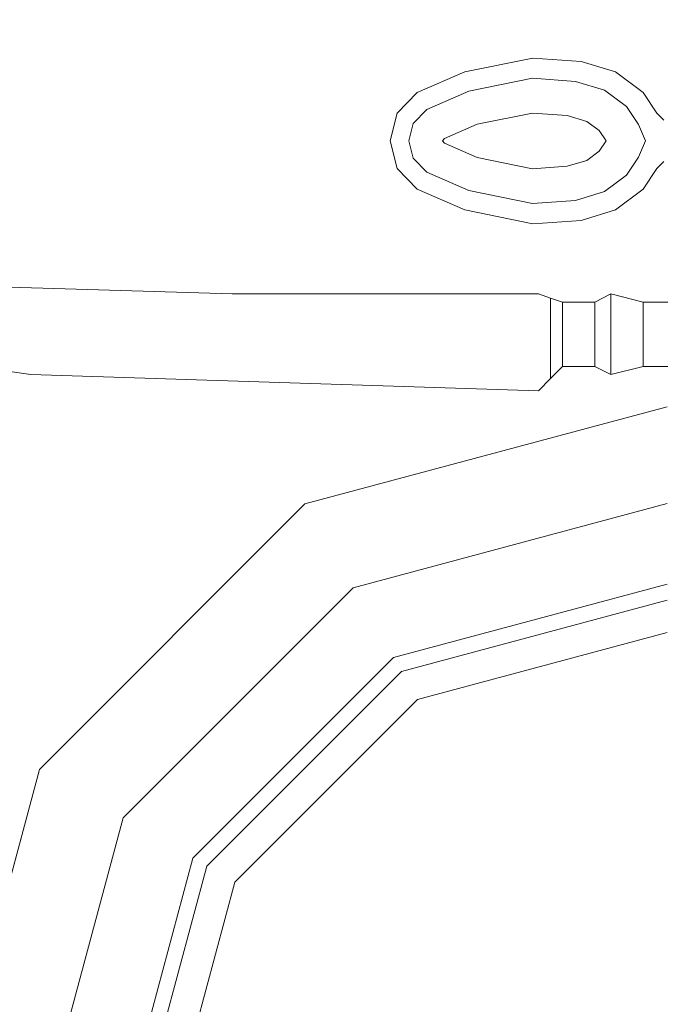
# Model space of a CAD drawing. Units: inches. Extents: x 375 to 1122, y 27 to 1069.
# Tile 62 of 155: x 734.823 to 739.718, y 304.063 to 311.585. Entities that reach past the tile are written whole.
import ezdxf

# ---------------------------------------------------------------- set-up
doc = ezdxf.new("R2010")
doc.units = ezdxf.units.IN
doc.layers.add('A-ANNO-DIMS', color=2, linetype='Continuous', lineweight=18)
doc.layers.add('Furniture', color=30, linetype='Continuous', lineweight=18)
doc.styles.get("Standard").update_dxf_attribs({"font": 'arial.ttf'})
doc.dimstyles.new('ISO-25', dxfattribs={"dimtxt": 12, "dimasz": 2.5, "dimexe": 1.5, "dimexo": 1.5, "dimtad": 1, "dimdec": 1, "dimlunit": 3, "dimtxsty": 'Standard', "dimblk": 'ARCHTICK', "dimcen": 2.5, "dimadec": 0, "dimazin": 0, "dimtfac": 1, "dimtdec": 1, "dimtmove": 0, "dimatfit": 3, "dimfxl": 1.5, "dimfxlon": 1, "dimarcsym": 0})

# ---------------------------------------------------------------- blocks, each defined once
blk = doc.blocks.new('A$C403C54AD')
for points, invisible_edges in [([(0.93398, 1.36607, -0.03581), (0.92167, 1.36607, -0.03581), (0.92167, 1.40455, -0.03427), (0.93398, 1.40455, -0.03427)], 4), ([(0.93398, 1.36607, -0.04504), (0.92167, 1.36607, -0.04504), (0.92167, 1.40455, -0.04658), (0.93398, 1.40455, -0.04658)], 4), ([(0.89484, 1.37003, -0.04027), (0.88693, 1.37003, -0.04027), (0.88561, 1.3687, -0.041), (0.89616, 1.3687, -0.041)], 5), ([(0.89484, 1.37003, -0.04236), (0.88693, 1.37003, -0.04236), (0.88561, 1.3687, -0.04315), (0.89616, 1.3687, -0.04315)], 5), ([(0.88693, 1.37003, -0.04236), (0.88693, 1.37003, -0.04027), (0.88561, 1.3687, -0.041), (0.88561, 1.3687, -0.04315)], 1), ([(0.89484, 1.37003, -0.04027), (0.89484, 1.37003, -0.04236), (0.89616, 1.3687, -0.04315), (0.89616, 1.3687, -0.041)], 1), ([(0.88774, 1.36518, -0.04424), (0.88561, 1.3687, -0.04315), (0.88165, 1.36608, -0.04195), (0.88434, 1.36289, -0.04423)], 5), ([(0.88774, 1.36518, -0.04292), (0.88561, 1.3687, -0.041), (0.88165, 1.36608, -0.04063), (0.88434, 1.36289, -0.04291)], 5), ([(0.88561, 1.3687, -0.04315), (0.89088, 1.3687, -0.04315), (0.89088, 1.36654, -0.04406), (0.88774, 1.36518, -0.04424)], 11), ([(0.88561, 1.3687, -0.041), (0.89088, 1.3687, -0.041), (0.89088, 1.36654, -0.04274), (0.88774, 1.36518, -0.04292)], 11), ([(0.89616, 1.3687, -0.04315), (0.89088, 1.3687, -0.04315), (0.89088, 1.36654, -0.04406), (0.89402, 1.36518, -0.04424)], 11), ([(0.89616, 1.3687, -0.041), (0.89088, 1.3687, -0.041), (0.89088, 1.36654, -0.04274), (0.89402, 1.36518, -0.04292)], 11), ([(0.89402, 1.36518, -0.04292), (0.89616, 1.3687, -0.041), (0.90012, 1.36608, -0.04063), (0.89743, 1.36289, -0.04291)], 5), ([(0.88165, 1.36608, -0.04195), (0.88434, 1.36289, -0.04423), (0.88119, 1.35867, -0.04406), (0.87769, 1.36082, -0.04147)], 5), ([(0.88165, 1.36608, -0.04063), (0.88434, 1.36289, -0.04291), (0.88119, 1.35867, -0.04274), (0.87769, 1.36082, -0.04015)], 5), ([(0.88774, 1.36518, -0.04424), (0.89088, 1.35902, -0.04627), (0.89088, 1.35902, -0.04627), (0.89088, 1.36654, -0.04406)], 5), ([(0.88774, 1.36518, -0.04292), (0.89088, 1.35902, -0.04495), (0.89088, 1.35902, -0.04495), (0.89088, 1.36654, -0.04274)], 5), ([(0.89402, 1.36518, -0.04424), (0.89088, 1.35902, -0.04627), (0.89088, 1.35902, -0.04627), (0.89088, 1.36654, -0.04406)], 5), ([(0.89402, 1.36518, -0.04292), (0.89088, 1.35902, -0.04495), (0.89088, 1.35902, -0.04495), (0.89088, 1.36654, -0.04274)], 5), ([(0.90012, 1.36608, -0.04195), (0.89743, 1.36289, -0.04423), (0.90058, 1.35867, -0.04406), (0.90408, 1.36082, -0.04147)], 5), ([(0.90012, 1.36608, -0.04063), (0.89743, 1.36289, -0.04291), (0.90058, 1.35867, -0.04274), (0.90408, 1.36082, -0.04015)], 5), ([(0.88892, 1.35767, -0.04647), (0.88434, 1.36289, -0.04423), (0.88774, 1.36518, -0.04424), (0.89088, 1.35902, -0.04627)], 5), ([(0.88892, 1.35767, -0.04515), (0.88434, 1.36289, -0.04291), (0.88774, 1.36518, -0.04292), (0.89088, 1.35902, -0.04495)], 5), ([(0.89284, 1.35767, -0.04647), (0.89743, 1.36289, -0.04423), (0.89402, 1.36518, -0.04424), (0.89088, 1.35902, -0.04627)], 5), ([(0.89284, 1.35767, -0.04515), (0.89743, 1.36289, -0.04291), (0.89402, 1.36518, -0.04292), (0.89088, 1.35902, -0.04495)], 5), ([(0.88119, 1.35867, -0.04406), (0.88715, 1.3553, -0.04638), (0.88892, 1.35767, -0.04647), (0.88434, 1.36289, -0.04423)], 5), ([(0.88119, 1.35867, -0.04274), (0.88715, 1.3553, -0.04506), (0.88892, 1.35767, -0.04515), (0.88434, 1.36289, -0.04291)], 5), ([(0.90058, 1.35867, -0.04406), (0.89462, 1.3553, -0.04638), (0.89284, 1.35767, -0.04647), (0.89743, 1.36289, -0.04423)], 5), ([(0.90058, 1.35867, -0.04274), (0.89462, 1.3553, -0.04506), (0.89284, 1.35767, -0.04515), (0.89743, 1.36289, -0.04291)], 5), ([(0.88119, 1.35867, -0.04274), (0.87769, 1.36082, -0.04015), (0.87571, 1.35422, -0.03974), (0.87953, 1.35316, -0.04222)], 5), ([(0.88119, 1.35867, -0.04406), (0.87769, 1.36082, -0.04147), (0.87571, 1.35422, -0.04106), (0.87953, 1.35316, -0.04354)], 5), ([(0.90058, 1.35867, -0.04274), (0.90408, 1.36082, -0.04015), (0.90606, 1.35422, -0.03974), (0.90224, 1.35316, -0.04222)], 5), ([(0.90058, 1.35867, -0.04406), (0.90408, 1.36082, -0.04147), (0.90606, 1.35422, -0.04106), (0.90224, 1.35316, -0.04354)], 5), ([(0.88604, 1.35158, -0.04614), (0.87953, 1.35316, -0.04354), (0.88119, 1.35867, -0.04406), (0.88715, 1.3553, -0.04638)], 5), ([(0.88604, 1.35158, -0.04482), (0.87953, 1.35316, -0.04222), (0.88119, 1.35867, -0.04274), (0.88715, 1.3553, -0.04506)], 5), ([(0.88892, 1.35767, -0.04647), (0.89284, 1.35767, -0.04647), (0.89088, 1.35902, -0.04627)], 1), ([(0.88892, 1.35767, -0.04515), (0.89284, 1.35767, -0.04515), (0.89088, 1.35902, -0.04495)], 1), ([(0.89573, 1.35158, -0.04482), (0.90224, 1.35316, -0.04222), (0.90058, 1.35867, -0.04274), (0.89462, 1.3553, -0.04506)], 5), ([(0.89462, 1.3553, -0.04638), (0.88715, 1.3553, -0.04638), (0.88892, 1.35767, -0.04647), (0.89284, 1.35767, -0.04647)], 5), ([(0.89462, 1.3553, -0.04506), (0.88715, 1.3553, -0.04506), (0.88892, 1.35767, -0.04515), (0.89284, 1.35767, -0.04515)], 5), ([(0.92167, 1.35684, -0.04504), (0.92167, 1.35684, -0.03581), (0.92167, 1.35068, -0.03581), (0.92167, 1.35068, -0.04504)], 4), ([(0.93398, 1.35068, -0.04504), (0.93398, 1.35068, -0.03581), (0.93398, 1.35684, -0.03581), (0.93398, 1.35684, -0.04504)], 1), ([(0.87571, 1.35422, -0.03974), (0.87953, 1.35316, -0.04222), (0.87893, 1.34491, -0.04133), (0.87505, 1.34501, -0.03888)], 5), ([(0.87571, 1.35422, -0.04106), (0.87953, 1.35316, -0.04354), (0.87893, 1.34491, -0.04265), (0.87505, 1.34501, -0.0402)], 5), ([(0.88604, 1.35158, -0.04614), (0.89573, 1.35158, -0.04614), (0.89462, 1.3553, -0.04638), (0.88715, 1.3553, -0.04638)], 5), ([(0.88604, 1.35158, -0.04482), (0.89573, 1.35158, -0.04482), (0.89462, 1.3553, -0.04506), (0.88715, 1.3553, -0.04506)], 5), ([(0.90606, 1.35422, -0.03974), (0.90224, 1.35316, -0.04222), (0.90283, 1.34491, -0.04133), (0.90672, 1.34501, -0.03888)], 5), ([(0.90606, 1.35422, -0.04106), (0.90224, 1.35316, -0.04354), (0.90283, 1.34491, -0.04265), (0.90672, 1.34501, -0.0402)], 5), ([(0.87893, 1.34491, -0.04265), (0.88556, 1.34497, -0.0452), (0.88604, 1.35158, -0.04614), (0.87953, 1.35316, -0.04354)], 5), ([(0.87893, 1.34491, -0.04133), (0.88556, 1.34497, -0.04388), (0.88604, 1.35158, -0.04482), (0.87953, 1.35316, -0.04222)], 5), ([(0.90283, 1.34491, -0.04265), (0.89621, 1.34497, -0.0452), (0.89573, 1.35158, -0.04614), (0.90224, 1.35316, -0.04354)], 5), ([(0.90283, 1.34491, -0.04133), (0.89621, 1.34497, -0.04388), (0.89573, 1.35158, -0.04482), (0.90224, 1.35316, -0.04222)], 5), ([(0.89621, 1.34497, -0.0452), (0.88556, 1.34497, -0.0452), (0.88604, 1.35158, -0.04614), (0.89573, 1.35158, -0.04614)], 5), ([(0.89621, 1.34497, -0.04388), (0.88556, 1.34497, -0.04388), (0.88604, 1.35158, -0.04482), (0.89573, 1.35158, -0.04482)], 5), ([(0.92167, 1.35068, -0.03581), (0.92167, 1.35068, -0.04504), (0.9209, 1.34837, -0.04196), (0.9209, 1.34837, -0.03888)], 5), ([(0.93629, 1.34837, -0.03888), (0.93629, 1.34837, -0.04196), (0.93398, 1.35068, -0.04504), (0.93398, 1.35068, -0.03581)], 5), ([(0.9386, 1.34606, -0.03965), (0.92013, 1.34606, -0.03965), (0.9209, 1.34837, -0.03888), (0.93629, 1.34837, -0.03888)], 1), ([(0.9386, 1.34606, -0.04119), (0.92013, 1.34606, -0.04119), (0.9209, 1.34837, -0.04196), (0.93629, 1.34837, -0.04196)], 1), ([(0.9209, 1.34837, -0.04196), (0.9209, 1.34837, -0.03888), (0.92013, 1.34606, -0.03965), (0.92013, 1.34606, -0.04119)], 5), ([(0.9386, 1.34606, -0.04119), (0.9386, 1.34606, -0.03965), (0.93629, 1.34837, -0.03888), (0.93629, 1.34837, -0.04196)], 5), ([(0.87893, 1.34491, -0.04265), (0.87505, 1.34501, -0.0402), (0.87769, 1.33198, -0.03816), (0.88139, 1.33278, -0.04067)], 5), ([(0.87893, 1.34491, -0.04133), (0.87505, 1.34501, -0.03888), (0.87769, 1.33198, -0.03684), (0.88139, 1.33278, -0.03935)], 5), ([(0.88771, 1.33436, -0.04216), (0.88139, 1.33278, -0.03935), (0.87893, 1.34491, -0.04133), (0.88556, 1.34497, -0.04388)], 5), ([(0.88771, 1.33436, -0.04348), (0.88139, 1.33278, -0.04067), (0.87893, 1.34491, -0.04265), (0.88556, 1.34497, -0.0452)], 5), ([(0.88771, 1.33436, -0.04216), (0.89406, 1.33436, -0.04216), (0.89621, 1.34497, -0.04388), (0.88556, 1.34497, -0.04388)], 5), ([(0.88771, 1.33436, -0.04348), (0.89406, 1.33436, -0.04348), (0.89621, 1.34497, -0.0452), (0.88556, 1.34497, -0.0452)], 5), ([(0.89406, 1.33436, -0.04216), (0.90038, 1.33278, -0.03935), (0.90283, 1.34491, -0.04133), (0.89621, 1.34497, -0.04388)], 5), ([(0.89406, 1.33436, -0.04348), (0.90038, 1.33278, -0.04067), (0.90283, 1.34491, -0.04265), (0.89621, 1.34497, -0.0452)], 5), ([(0.90283, 1.34491, -0.04265), (0.90672, 1.34501, -0.0402), (0.90408, 1.33198, -0.03816), (0.90038, 1.33278, -0.04067)], 5), ([(0.90283, 1.34491, -0.04133), (0.90672, 1.34501, -0.03888), (0.90408, 1.33198, -0.03684), (0.90038, 1.33278, -0.03935)], 5), ([(0.92013, 1.28757, -0.03965), (0.93552, 1.24909, -0.03965), (0.9386, 1.34606, -0.03965), (0.92013, 1.34606, -0.03965)], 5), ([(0.92013, 1.28757, -0.04119), (0.93552, 1.24909, -0.04119), (0.9386, 1.34606, -0.04119), (0.92013, 1.34606, -0.04119)], 5), ([(0.92013, 1.34606, -0.03965), (0.92013, 1.34606, -0.04119), (0.92013, 1.28757, -0.04119), (0.92013, 1.28757, -0.03965)], 5), ([(0.93552, 1.24909, -0.04119), (0.93552, 1.24909, -0.03965), (0.9386, 1.34606, -0.03965), (0.9386, 1.34606, -0.04119)], 5), ([(0.8849, 1.32476, -0.03896), (0.89045, 1.32814, -0.04186), (0.88771, 1.33436, -0.04348), (0.88139, 1.33278, -0.04067)], 5), ([(0.8849, 1.32476, -0.03764), (0.89045, 1.32814, -0.04054), (0.88771, 1.33436, -0.04216), (0.88139, 1.33278, -0.03935)], 5), ([(0.89132, 1.32814, -0.04186), (0.89045, 1.32814, -0.04186), (0.88771, 1.33436, -0.04348), (0.89406, 1.33436, -0.04348)], 5), ([(0.89132, 1.32814, -0.04054), (0.89045, 1.32814, -0.04054), (0.88771, 1.33436, -0.04216), (0.89406, 1.33436, -0.04216)], 5), ([(0.89687, 1.32476, -0.03896), (0.89132, 1.32814, -0.04186), (0.89406, 1.33436, -0.04348), (0.90038, 1.33278, -0.04067)], 5), ([(0.89687, 1.32476, -0.03764), (0.89132, 1.32814, -0.04054), (0.89406, 1.33436, -0.04216), (0.90038, 1.33278, -0.03935)], 5), ([(0.87769, 1.33198, -0.03816), (0.88139, 1.33278, -0.04067), (0.8849, 1.32476, -0.03896), (0.88165, 1.32291, -0.03632)], 5), ([(0.87769, 1.33198, -0.03684), (0.88139, 1.33278, -0.03935), (0.8849, 1.32476, -0.03764), (0.88165, 1.32291, -0.035)], 5), ([(0.90408, 1.33198, -0.03816), (0.90038, 1.33278, -0.04067), (0.89687, 1.32476, -0.03896), (0.90012, 1.32291, -0.03632)], 5), ([(0.90408, 1.33198, -0.03684), (0.90038, 1.33278, -0.03935), (0.89687, 1.32476, -0.03764), (0.90012, 1.32291, -0.035)], 5), ([(0.89045, 1.32814, -0.04054), (0.88758, 1.32213, -0.03709), (0.8849, 1.32476, -0.03764), (0.89045, 1.32814, -0.04054)], 5), ([(0.89045, 1.32814, -0.04186), (0.88758, 1.32213, -0.03841), (0.8849, 1.32476, -0.03896), (0.89045, 1.32814, -0.04186)], 5), ([(0.89088, 1.32132, -0.0369), (0.89088, 1.32772, -0.0404), (0.89045, 1.32814, -0.04054), (0.88758, 1.32213, -0.03709)], 5), ([(0.89088, 1.32132, -0.03822), (0.89088, 1.32772, -0.04172), (0.89045, 1.32814, -0.04186), (0.88758, 1.32213, -0.03841)], 5), ([(0.89088, 1.32772, -0.0404), (0.89045, 1.32814, -0.04054), (0.89132, 1.32814, -0.04054), (0.89088, 1.32772, -0.0404)], 2), ([(0.89088, 1.32772, -0.04172), (0.89045, 1.32814, -0.04186), (0.89132, 1.32814, -0.04186), (0.89088, 1.32772, -0.04172)], 2), ([(0.89088, 1.32132, -0.0369), (0.89088, 1.32772, -0.0404), (0.89132, 1.32814, -0.04054), (0.89419, 1.32213, -0.03709)], 5), ([(0.89088, 1.32132, -0.03822), (0.89088, 1.32772, -0.04172), (0.89132, 1.32814, -0.04186), (0.89419, 1.32213, -0.03841)], 5), ([(0.89132, 1.32814, -0.04054), (0.89419, 1.32213, -0.03709), (0.89687, 1.32476, -0.03764), (0.89132, 1.32814, -0.04054)], 5), ([(0.89132, 1.32814, -0.04186), (0.89419, 1.32213, -0.03841), (0.89687, 1.32476, -0.03896), (0.89132, 1.32814, -0.04186)], 5), ([(0.8849, 1.32476, -0.03896), (0.88165, 1.32291, -0.03632), (0.88561, 1.31907, -0.03523), (0.88758, 1.32213, -0.03841)], 5), ([(0.8849, 1.32476, -0.03764), (0.88165, 1.32291, -0.035), (0.88561, 1.31907, -0.03391), (0.88758, 1.32213, -0.03709)], 5), ([(0.89687, 1.32476, -0.03896), (0.90012, 1.32291, -0.03632), (0.89616, 1.31907, -0.03523), (0.89419, 1.32213, -0.03841)], 5), ([(0.89687, 1.32476, -0.03764), (0.90012, 1.32291, -0.035), (0.89616, 1.31907, -0.03391), (0.89419, 1.32213, -0.03709)], 5), ([(0.88561, 1.31907, -0.03523), (0.88758, 1.32213, -0.03841), (0.89088, 1.32132, -0.03822), (0.89088, 1.31776, -0.03505)], 5), ([(0.88561, 1.31907, -0.03391), (0.88758, 1.32213, -0.03709), (0.89088, 1.32132, -0.0369), (0.89088, 1.31776, -0.03373)], 5), ([(0.89616, 1.31907, -0.03523), (0.89419, 1.32213, -0.03841), (0.89088, 1.32132, -0.03822), (0.89088, 1.31776, -0.03505)], 5), ([(0.89616, 1.31907, -0.03391), (0.89419, 1.32213, -0.03709), (0.89088, 1.32132, -0.0369), (0.89088, 1.31776, -0.03373)], 5), ([(0.93398, 1.23832, -0.03965), (0.91859, 1.23832, -0.03965), (0.92013, 1.28757, -0.03965), (0.93552, 1.24909, -0.03965)], 5), ([(0.93398, 1.23832, -0.04119), (0.91859, 1.23832, -0.04119), (0.92013, 1.28757, -0.04119), (0.93552, 1.24909, -0.04119)], 5), ([(0.92013, 1.28757, -0.04119), (0.92013, 1.28757, -0.03965), (0.91859, 1.23832, -0.03965), (0.91859, 1.23832, -0.04119)], 5), ([(0.93398, 1.23832, -0.03965), (0.93398, 1.23832, -0.04119), (0.93552, 1.24909, -0.04119), (0.93552, 1.24909, -0.03965)], 5)]:
    blk.add_3dface(points, dxfattribs=dict(invisible_edges=invisible_edges))
for points in [[(0.92167, 1.40455, -0.03427), (0.92167, 1.40455, -0.04658), (0.92167, 1.36607, -0.04504), (0.92167, 1.36607, -0.03581)], [(0.93398, 1.36607, -0.03581), (0.93398, 1.36607, -0.04504), (0.93398, 1.40455, -0.04658), (0.93398, 1.40455, -0.03427)], [(0.88561, 1.3687, -0.04315), (0.88561, 1.3687, -0.041), (0.88165, 1.36608, -0.04063), (0.88165, 1.36608, -0.04195)], [(0.90012, 1.36608, -0.04195), (0.90012, 1.36608, -0.04063), (0.89616, 1.3687, -0.041), (0.89616, 1.3687, -0.04315)], [(0.88165, 1.36608, -0.04063), (0.88165, 1.36608, -0.04195), (0.87769, 1.36082, -0.04147), (0.87769, 1.36082, -0.04015)], [(0.90408, 1.36082, -0.04015), (0.90408, 1.36082, -0.04147), (0.90012, 1.36608, -0.04195), (0.90012, 1.36608, -0.04063)], [(0.92013, 1.35991, -0.03427), (0.93552, 1.35991, -0.03427), (0.93398, 1.36607, -0.03581), (0.92167, 1.36607, -0.03581)], [(0.92013, 1.35991, -0.04658), (0.93552, 1.35991, -0.04658), (0.93398, 1.36607, -0.04504), (0.92167, 1.36607, -0.04504)], [(0.92167, 1.36607, -0.04504), (0.92167, 1.36607, -0.03581), (0.92013, 1.35991, -0.03427), (0.92013, 1.35991, -0.04658)], [(0.93552, 1.35991, -0.04658), (0.93552, 1.35991, -0.03427), (0.93398, 1.36607, -0.03581), (0.93398, 1.36607, -0.04504)], [(0.87769, 1.36082, -0.04147), (0.87769, 1.36082, -0.04015), (0.87571, 1.35422, -0.03974), (0.87571, 1.35422, -0.04106)], [(0.90606, 1.35422, -0.04106), (0.90606, 1.35422, -0.03974), (0.90408, 1.36082, -0.04015), (0.90408, 1.36082, -0.04147)], [(0.93398, 1.35684, -0.03581), (0.92167, 1.35684, -0.03581), (0.92013, 1.35991, -0.03427), (0.93552, 1.35991, -0.03427)], [(0.93398, 1.35684, -0.04504), (0.92167, 1.35684, -0.04504), (0.92013, 1.35991, -0.04658), (0.93552, 1.35991, -0.04658)], [(0.92013, 1.35991, -0.03427), (0.92013, 1.35991, -0.04658), (0.92167, 1.35684, -0.04504), (0.92167, 1.35684, -0.03581)], [(0.93398, 1.35684, -0.03581), (0.93398, 1.35684, -0.04504), (0.93552, 1.35991, -0.04658), (0.93552, 1.35991, -0.03427)], [(0.92167, 1.35068, -0.03581), (0.93398, 1.35068, -0.03581), (0.93398, 1.35684, -0.03581), (0.92167, 1.35684, -0.03581)], [(0.92167, 1.35068, -0.04504), (0.93398, 1.35068, -0.04504), (0.93398, 1.35684, -0.04504), (0.92167, 1.35684, -0.04504)], [(0.87571, 1.35422, -0.03974), (0.87571, 1.35422, -0.04106), (0.87505, 1.34501, -0.0402), (0.87505, 1.34501, -0.03888)], [(0.90672, 1.34501, -0.0402), (0.90672, 1.34501, -0.03888), (0.90606, 1.35422, -0.03974), (0.90606, 1.35422, -0.04106)], [(0.93629, 1.34837, -0.03888), (0.9209, 1.34837, -0.03888), (0.92167, 1.35068, -0.03581), (0.93398, 1.35068, -0.03581)], [(0.93629, 1.34837, -0.04196), (0.9209, 1.34837, -0.04196), (0.92167, 1.35068, -0.04504), (0.93398, 1.35068, -0.04504)], [(0.87505, 1.34501, -0.0402), (0.87505, 1.34501, -0.03888), (0.87769, 1.33198, -0.03684), (0.87769, 1.33198, -0.03816)], [(0.90408, 1.33198, -0.03684), (0.90408, 1.33198, -0.03816), (0.90672, 1.34501, -0.0402), (0.90672, 1.34501, -0.03888)], [(0.87769, 1.33198, -0.03684), (0.87769, 1.33198, -0.03816), (0.88165, 1.32291, -0.03632), (0.88165, 1.32291, -0.035)], [(0.90012, 1.32291, -0.03632), (0.90012, 1.32291, -0.035), (0.90408, 1.33198, -0.03684), (0.90408, 1.33198, -0.03816)], [(0.88165, 1.32291, -0.03632), (0.88165, 1.32291, -0.035), (0.88561, 1.31907, -0.03391), (0.88561, 1.31907, -0.03523)], [(0.89616, 1.31907, -0.03391), (0.89616, 1.31907, -0.03523), (0.90012, 1.32291, -0.03632), (0.90012, 1.32291, -0.035)], [(0.88561, 1.31907, -0.03391), (0.88561, 1.31907, -0.03523), (0.89088, 1.31776, -0.03505), (0.89088, 1.31776, -0.03373)], [(0.89088, 1.31776, -0.03505), (0.89088, 1.31776, -0.03373), (0.89616, 1.31907, -0.03391), (0.89616, 1.31907, -0.03523)]]:
    blk.add_3dface(points)
at = {"linetype": 'ByBlock', "invisible_edges": 5}
for points in [[(0.94168, 1.37069, -0.02349), (0.96015, 1.37069, -0.02349), (0.97623, 1.31066, -0.02349), (0.96024, 1.30143, -0.02349)], [(0.97554, 1.37069, -0.03734), (0.94168, 1.37069, -0.02811), (0.96024, 1.30143, -0.02811), (0.98956, 1.31836, -0.03734)], [(0.96015, 1.37069, -0.02349), (0.97862, 1.37069, -0.02965), (0.99223, 1.3199, -0.02965), (0.97623, 1.31066, -0.02349)], [(0.98477, 1.37069, -0.04658), (0.97554, 1.37069, -0.03734), (0.98956, 1.31836, -0.03734), (0.99756, 1.32297, -0.04658)], [(0.97862, 1.37069, -0.02965), (1.0802, 1.37069, -0.02965), (1.0802, 1.37069, -0.02965), (0.99223, 1.3199, -0.02965)], [(0.99223, 1.3199, -0.02965), (1.0802, 1.37069, -0.02965), (1.0802, 1.37069, -0.02965), (1.02941, 1.28271, -0.02965)], [(1.02941, 1.28271, -0.02965), (1.0802, 1.37069, -0.02965), (1.0802, 1.37069, -0.02965), (1.0802, 1.2691, -0.02965)], [(0.99756, 1.32297, -0.04658), (0.98956, 1.31836, -0.03734), (1.02787, 1.28005, -0.03734), (1.03249, 1.28804, -0.04658)], [(0.97623, 1.31066, -0.02349), (0.99223, 1.3199, -0.02965), (1.02941, 1.28271, -0.02965), (1.02018, 1.26672, -0.02349)], [(0.98956, 1.31836, -0.03734), (0.96024, 1.30143, -0.02811), (1.01094, 1.25072, -0.02811), (1.02787, 1.28005, -0.03734)], [(0.96024, 1.30143, -0.02349), (0.97623, 1.31066, -0.02349), (1.02018, 1.26672, -0.02349), (1.01094, 1.25072, -0.02349)], [(1.03249, 1.28804, -0.04658), (1.02787, 1.28005, -0.03734), (1.0802, 1.26602, -0.03734), (1.0802, 1.27526, -0.04658)], [(1.02018, 1.26672, -0.02349), (1.02941, 1.28271, -0.02965), (1.0802, 1.2691, -0.02965), (1.0802, 1.25063, -0.02349)], [(1.02787, 1.28005, -0.03734), (1.01094, 1.25072, -0.02811), (1.0802, 1.23216, -0.02811), (1.0802, 1.26602, -0.03734)], [(1.01094, 1.25072, -0.02349), (1.02018, 1.26672, -0.02349), (1.0802, 1.25063, -0.02349), (1.0802, 1.23216, -0.02349)]]:
    blk.add_3dface(points, dxfattribs=at)
at = {"linetype": 'ByBlock'}
for points in [[(0.94168, 1.37069, -0.02811), (0.94168, 1.37069, -0.02349), (0.96024, 1.30143, -0.02349), (0.96024, 1.30143, -0.02811)], [(0.96024, 1.30143, -0.02811), (0.96024, 1.30143, -0.02349), (1.01094, 1.25072, -0.02349), (1.01094, 1.25072, -0.02811)], [(1.01094, 1.25072, -0.02811), (1.01094, 1.25072, -0.02349), (1.0802, 1.23216, -0.02349), (1.0802, 1.23216, -0.02811)]]:
    blk.add_3dface(points, dxfattribs=at)
blk = doc.blocks.new('_ArchTick')
at = {"color": 0, "linetype": 'ByBlock', "const_width": 0.15}
blk.add_lwpolyline([(-0.5, -0.5), (0.5, 0.5)], dxfattribs=at)
blk = doc.blocks.new('*D94')
at = {"layer": 'A-ANNO-DIMS', "color": 0, "lineweight": -2, "transparency": 16777216}
for p, q in [((734.0073, 117.5277), (734.0073, 114.5277)), ((773.0073, 117.5277), (773.0073, 114.5277)), ((734.0073, 116.0277), (773.0073, 116.0277))]:
    blk.add_line(p, q, dxfattribs=at)
at = {"layer": 'Defpoints', "color": 0, "transparency": 16777216}
for p in [(734.0073, 667.5277), (773.0073, 667.5277), (773.0073, 116.0277)]:
    blk.add_point(p, dxfattribs=at)
at = {"layer": 'A-ANNO-DIMS', "color": 0, "lineweight": -2, "transparency": 16777216, "xscale": 2.5, "yscale": 2.5, "zscale": 2.5, "rotation": 180}
blk.add_blockref('_ArchTick', (734.0073, 116.0277), dxfattribs=at)
at = {"layer": 'A-ANNO-DIMS', "color": 0, "lineweight": -2, "transparency": 16777216, "xscale": 2.5, "yscale": 2.5, "zscale": 2.5}
blk.add_blockref('_ArchTick', (773.0073, 116.0277), dxfattribs=at)
at = {"layer": 'A-ANNO-DIMS', "color": 0, "transparency": 16777216, "insert": (753.5073, 122.7837), "char_height": 12, "attachment_point": 5}
blk.add_mtext('3\'-3"', dxfattribs=at)

msp = doc.modelspace()

# ---------------------------------------------------------------- block references
at = {"layer": 'Furniture', "xscale": 39.9918517141215, "yscale": 39.9918517141215, "zscale": 39.9918517141215, "rotation": 270}
msp.add_blockref('A$C403C54AD', (684.9549, 346.2875, 0.024), dxfattribs=at)

# ---------------------------------------------------------------- dimensions: what is measured, and where the dimension line sits
at = {"layer": 'A-ANNO-DIMS'}
dim = msp.add_linear_dim(base=(773.0073, 116.0277), p1=(734.0073, 667.5277), p2=(773.0073, 667.5277), dimstyle='ISO-25', override={"dimdec": 1, "dimlfac": 1, "dimrnd": 0, "dimzin": 1, "dimdsep": 46, "dimlunit": 4, "dimfrac": 2}, dxfattribs=at)
dim.commit()
dim.dimension.update_dxf_attribs({"geometry": '*D94', "text_midpoint": (753.5073, 122.7837)})

doc.saveas('drawing.dxf')
